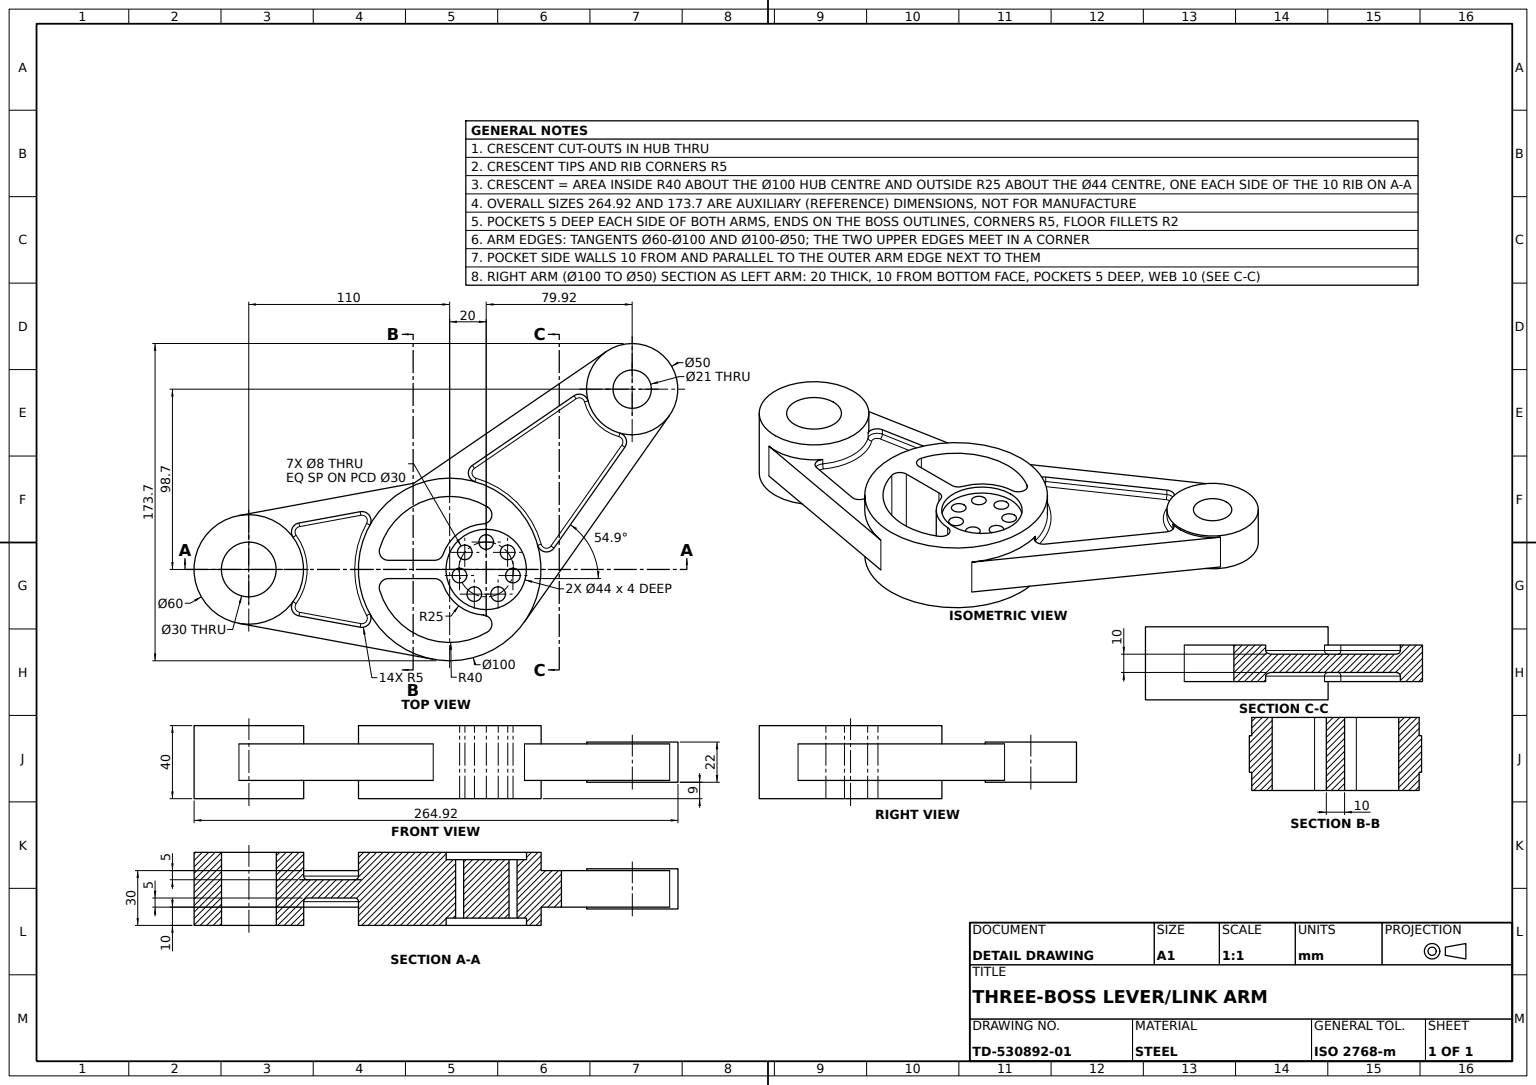
from build123d import *

# Parameters (mm, degrees)
BELLCRANK_PROFILE_SKETCH_R   = 50
BELLCRANK_PROFILE_SKETCH_R_2 = 22
BELLCRANK_BODY_DEPTH         = 20
HUB_HOLE_CIRCLE_SKETCH_R     = 22
HUB_HOLE_CIRCLE_SKETCH_R_2   = 4
HUB_HOLES_7X_8_DEPTH         = 16
ARM_A_WEB_SKETCH_R           = 25
ARM_A_WEB_SKETCH_R_2         = 10.5
ARM_A_WEB_DEPTH              = 11
ARM_A_POCKET_DEPTH           = 10
ARM_A_INNER_POCKET_DEPTH     = 5
ARM_A_POCKET_FILLETS_R2_R    = 2
ARM_B_SKETCH_R               = 30
ARM_B_SKETCH_R_2             = 15
ARM_B_DEPTH                  = 20
ARM_B_POCKET_DEPTH           = 10
ARM_B_INNER_POCKET_DEPTH     = 5
ARM_B_POCKET_FILLETS_R2_R    = 2


with BuildPart() as part:
    # Bellcrank Profile Sketch → Bellcrank Body (new, symmetric)
    with BuildSketch(Plane(origin=(0, 0, 0), x_dir=(1, 0, 0), z_dir=(0, 1, 0))):
        with Locations(Location((0, 0, 0), (0, 0, 270))):
            Circle(BELLCRANK_PROFILE_SKETCH_R)
        with Locations(Location((20, 0, 0), (0, 0, 270))):
            Circle(BELLCRANK_PROFILE_SKETCH_R_2, mode=Mode.SUBTRACT)
        with BuildLine():
            Line((-8.284271247, 5), (-33.541019662, 5))
            ThreePointArc((-33.541019662, 5), (-37.549938291, 7.011928477), (-38.3325939, 11.428571429))
            ThreePointArc((-38.3325939, 11.428571429), (-14.403072902, 37.316906235), (20.714285714, 34.218684477))
            ThreePointArc((20.714285714, 34.218684477), (22.980616225, 28.748457023), (18.4375, 24.951124098))
            ThreePointArc((18.4375, 24.951124098), (4.935099668, 19.951159815), (-3.57022604, 8.333333333))
            ThreePointArc((-3.57022604, 8.333333333), (-5.397519902, 5.917517095), (-8.284271247, 5))
        make_face(mode=Mode.SUBTRACT)
        with BuildLine():
            Line((-8.284271247, -5), (-33.541019662, -5))
            ThreePointArc((-33.541019662, -5), (-37.549938291, -7.011928477), (-38.3325939, -11.428571429))
            ThreePointArc((-38.3325939, -11.428571429), (-14.403072902, -37.316906235), (20.714285714, -34.218684477))
            ThreePointArc((20.714285714, -34.218684477), (22.980616225, -28.748457023), (18.4375, -24.951124098))
            ThreePointArc((18.4375, -24.951124098), (4.935099668, -19.951159815), (-3.57022604, -8.333333333))
            ThreePointArc((-3.57022604, -8.333333333), (-5.397519902, -5.917517095), (-8.284271247, -5))
        make_face(mode=Mode.SUBTRACT)
    extrude(amount=BELLCRANK_BODY_DEPTH, both=True)

    # Hub Hole Circle Sketch → Hub Holes 7x_8 (add, symmetric)
    with BuildSketch(Plane(origin=(0, 0, 0), x_dir=(1, 0, 0), z_dir=(0, 1, 0))):
        with Locations(Location((20, 0, 0), (0, 0, 270))):
            Circle(HUB_HOLE_CIRCLE_SKETCH_R)
        with Locations(Location((20, 15, 0), (0, 0, 270))):
            Circle(HUB_HOLE_CIRCLE_SKETCH_R_2, mode=Mode.SUBTRACT)
        with Locations(Location((31.727472237, 9.352347028, 0), (0, 0, 270))):
            Circle(HUB_HOLE_CIRCLE_SKETCH_R_2, mode=Mode.SUBTRACT)
        with Locations(Location((34.623918683, -3.337814009, 0), (0, 0, 270))):
            Circle(HUB_HOLE_CIRCLE_SKETCH_R_2, mode=Mode.SUBTRACT)
        with Locations(Location((26.508256087, -13.514533019, 0), (0, 0, 270))):
            Circle(HUB_HOLE_CIRCLE_SKETCH_R_2, mode=Mode.SUBTRACT)
        with Locations(Location((13.491743913, -13.514533019, 0), (0, 0, 270))):
            Circle(HUB_HOLE_CIRCLE_SKETCH_R_2, mode=Mode.SUBTRACT)
        with Locations(Location((5.376081317, -3.337814009, 0), (0, 0, 270))):
            Circle(HUB_HOLE_CIRCLE_SKETCH_R_2, mode=Mode.SUBTRACT)
        with Locations(Location((8.272527763, 9.352347028, 0), (0, 0, 270))):
            Circle(HUB_HOLE_CIRCLE_SKETCH_R_2, mode=Mode.SUBTRACT)
    extrude(amount=HUB_HOLES_7X_8_DEPTH, both=True)



with BuildPart() as body_2:
    # Arm A Web Sketch → Arm A Web (new, symmetric)
    with BuildSketch(Plane(origin=(0, 0, 0), x_dir=(1, 0, 0), z_dir=(0, 1, 0))):
        with Locations(Location((99.923689663, 98.697537105, 0), (0, 0, 270))):
            Circle(ARM_A_WEB_SKETCH_R)
        with Locations(Location((99.923689663, 98.697537105, 0), (0, 0, 270))):
            Circle(ARM_A_WEB_SKETCH_R_2, mode=Mode.SUBTRACT)
    extrude(amount=ARM_A_WEB_DEPTH, both=True)


with BuildPart() as part_1:
    add(part.part)

    add(body_2.part)  # Arm A Pocket merges body 2
    # Arm A Pocket Sketch → Arm A Pocket (add, symmetric)
    with BuildSketch(Plane(origin=(0, 0, 0), x_dir=(1, 0, 0), z_dir=(0, 1, 0))):
        with BuildLine():
            ThreePointArc((57.121474807, 11.710555748), (52.174454283, 9.659478884), (48.209768815, 13.2596452))
            ThreePointArc((48.209768815, 13.2596452), (49.261308362, -8.562914134), (40.907291105, -28.750539725))
            Line((40.907291105, -28.750539725), (120.377335216, 84.322267243))
            ThreePointArc((120.377335216, 84.322267243), (108.324455399, 75.151260647), (93.188437113, 74.621898524))
            ThreePointArc((93.188437113, 74.621898524), (96.550641894, 71.486923955), (95.932115713, 66.931716835))
            Line((95.932115713, 66.931716835), (57.121474807, 11.710555748))
        make_face()
        with BuildLine():
            Line((85.802039648, 119.327103287), (-28.243300031, 41.259132363))
            ThreePointArc((-28.243300031, 41.259132363), (-7.954072951, 49.363273023), (13.853840649, 48.042388567))
            ThreePointArc((13.853840649, 48.042388567), (10.302897412, 52.051220129), (12.414894711, 56.97254066))
            Line((12.414894711, 56.97254066), (68.11100983, 95.098453634))
            ThreePointArc((68.11100983, 95.098453634), (72.673506196, 95.660693306), (75.766731472, 92.260039849))
            ThreePointArc((75.766731472, 92.260039849), (76.48292512, 107.388368921), (85.802039648, 119.327103287))
        make_face()
    extrude(amount=ARM_A_POCKET_DEPTH, both=True)

    # Sketch4_3 → Arm A Inner Pocket (add, symmetric)
    with BuildSketch(Plane(origin=(0, 0, 0), x_dir=(1, 0, 0), z_dir=(0, 1, 0))):
        with BuildLine():
            ThreePointArc((93.188437113, 74.621898524), (96.550641894, 71.486923955), (95.932115713, 66.931716835))
            Line((95.932115713, 66.931716835), (57.121474807, 11.710555748))
            ThreePointArc((57.121474807, 11.710555748), (52.174454283, 9.659478884), (48.209768815, 13.2596452))
            ThreePointArc((48.209768815, 13.2596452), (35.572921077, 35.136409692), (13.853840649, 48.042388567))
            ThreePointArc((13.853840649, 48.042388567), (10.302897412, 52.051220129), (12.414894711, 56.97254066))
            Line((12.414894711, 56.97254066), (68.11100983, 95.098453634))
            ThreePointArc((68.11100983, 95.098453634), (72.673506196, 95.660693306), (75.766731472, 92.260039849))
            ThreePointArc((75.766731472, 92.260039849), (82.137229125, 81.129332259), (93.188437113, 74.621898524))
        make_face()
    extrude(amount=ARM_A_INNER_POCKET_DEPTH, both=True)

    # Arm A Pocket Fillets R2
    arm_a_pocket_fillets_r2_edges = [part_1.edges().sort_by_distance(p)[0] for p in [
        (96.550641894, 5, -71.486923955),
        (82.137229125, 5, -81.129332259),
        (72.673506196, -5, -95.660693306),
        (40.262952271, 5, -76.035497147),
        (10.302897412, 5, -52.051220129),
        (35.572921077, 5, -35.136409692),
        (52.174454283, 5, -9.659478884),
        (76.52679526, -5, -39.321136292),
        (72.673506196, 5, -95.660693306),
        (76.52679526, 5, -39.321136292),
        (96.550641894, -5, -71.486923955),
        (52.174454283, -5, -9.659478884),
        (35.572921077, -5, -35.136409692),
        (10.302897412, -5, -52.051220129),
        (40.262952271, -5, -76.035497147),
        (82.137229125, -5, -81.129332259),
    ]]
    fillet(arm_a_pocket_fillets_r2_edges, radius=ARM_A_POCKET_FILLETS_R2_R)



with BuildPart() as body_2_2:
    # Arm B Sketch → Arm B (new, symmetric)
    with BuildSketch(Plane(origin=(0, 0, 0), x_dir=(1, 0, 0), z_dir=(0, 1, 0))):
        with Locations(Location((-110, 0, 0), (0, 0, 270))):
            Circle(ARM_B_SKETCH_R)
        with Locations(Location((-110, 0, 0), (0, 0, 270))):
            Circle(ARM_B_SKETCH_R_2, mode=Mode.SUBTRACT)
    extrude(amount=ARM_B_DEPTH, both=True)


with BuildPart() as part_2:
    add(part_1.part)

    add(body_2_2.part)  # Arm B Pocket merges body 2 2
    # Arm B Pocket Sketch → Arm B Pocket (add, symmetric)
    with BuildSketch(Plane(origin=(0, 0, 0), x_dir=(1, 0, 0), z_dir=(0, 1, 0))):
        with BuildLine():
            ThreePointArc((-82.540670225, -25.416239066), (-86.272845666, -22.359321946), (-85.684210842, -17.57106706))
            ThreePointArc((-85.684210842, -17.57106706), (-98.841537744, -27.847598103), (-115.454545455, -29.499964981))
            Line((-115.454545455, -29.499964981), (-9.090909091, -49.166608302))
            ThreePointArc((-9.090909091, -49.166608302), (-29.187748892, -40.596493871), (-43.71171539, -24.275212412))
            ThreePointArc((-43.71171539, -24.275212412), (-44.023237542, -29.621508542), (-48.991977838, -31.619394483))
            Line((-48.991977838, -31.619394483), (-82.540670225, -25.416239066))
        make_face()
        with BuildLine():
            Line((-9.090909091, 49.166608302), (-115.454545455, 29.499964981))
            ThreePointArc((-115.454545455, 29.499964981), (-98.841537744, 27.847598103), (-85.684210842, 17.57106706))
            ThreePointArc((-85.684210842, 17.57106706), (-86.272845666, 22.359321946), (-82.540670225, 25.416239066))
            Line((-82.540670225, 25.416239066), (-48.991977838, 31.619394483))
            ThreePointArc((-48.991977838, 31.619394483), (-44.023237542, 29.621508542), (-43.71171539, 24.275212412))
            ThreePointArc((-43.71171539, 24.275212412), (-29.187748892, 40.596493871), (-9.090909091, 49.166608302))
        make_face()
    extrude(amount=ARM_B_POCKET_DEPTH, both=True)

    # Sketch7_4 → Arm B Inner Pocket (add, symmetric)
    with BuildSketch(Plane(origin=(0, 0, 0), x_dir=(1, 0, 0), z_dir=(0, 1, 0))):
        with BuildLine():
            Line((-82.540670225, 25.416239066), (-48.991977838, 31.619394483))
            ThreePointArc((-48.991977838, 31.619394483), (-44.023237542, 29.621508542), (-43.71171539, 24.275212412))
            ThreePointArc((-43.71171539, 24.275212412), (-50, 0), (-43.71171539, -24.275212412))
            ThreePointArc((-43.71171539, -24.275212412), (-44.023237542, -29.621508542), (-48.991977838, -31.619394483))
            Line((-48.991977838, -31.619394483), (-82.540670225, -25.416239066))
            ThreePointArc((-82.540670225, -25.416239066), (-86.272845666, -22.359321946), (-85.684210842, -17.57106706))
            ThreePointArc((-85.684210842, -17.57106706), (-80, 0), (-85.684210842, 17.57106706))
            ThreePointArc((-85.684210842, 17.57106706), (-86.272845666, 22.359321946), (-82.540670225, 25.416239066))
        make_face()
    extrude(amount=ARM_B_INNER_POCKET_DEPTH, both=True)

    # Arm B Pocket Fillets R2
    arm_b_pocket_fillets_r2_edges = [part_2.edges().sort_by_distance(p)[0] for p in [
        (-65.766324032, 5, -28.517816775),
        (-86.272845666, -5, -22.359321946),
        (-80, 5, 0),
        (-86.272845666, -5, 22.359321946),
        (-65.766324032, -5, 28.517816775),
        (-44.023237542, -5, 29.621508542),
        (-50, 5, 0),
        (-44.023237542, -5, -29.621508542),
        (-86.272845666, 5, -22.359321946),
        (-86.272845666, 5, 22.359321946),
        (-65.766324032, 5, 28.517816775),
        (-44.023237542, 5, 29.621508542),
        (-44.023237542, 5, -29.621508542),
        (-65.766324032, -5, -28.517816775),
        (-50, -5, 0),
        (-80, -5, 0),
    ]]
    fillet(arm_b_pocket_fillets_r2_edges, radius=ARM_B_POCKET_FILLETS_R2_R)


solid = part_2.part
